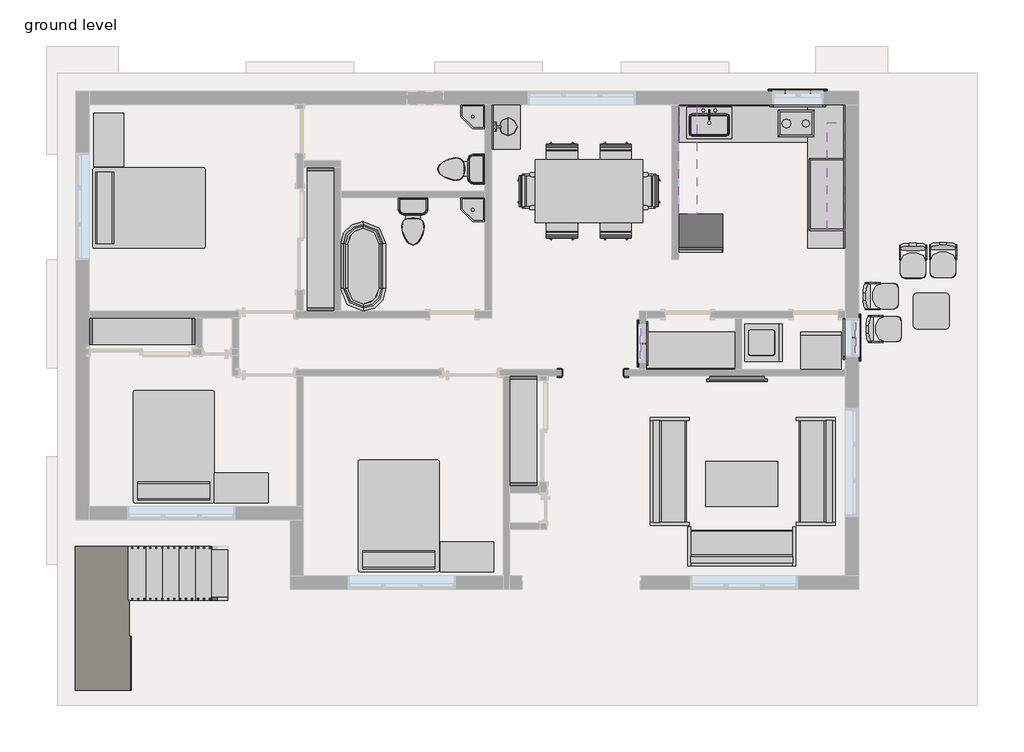
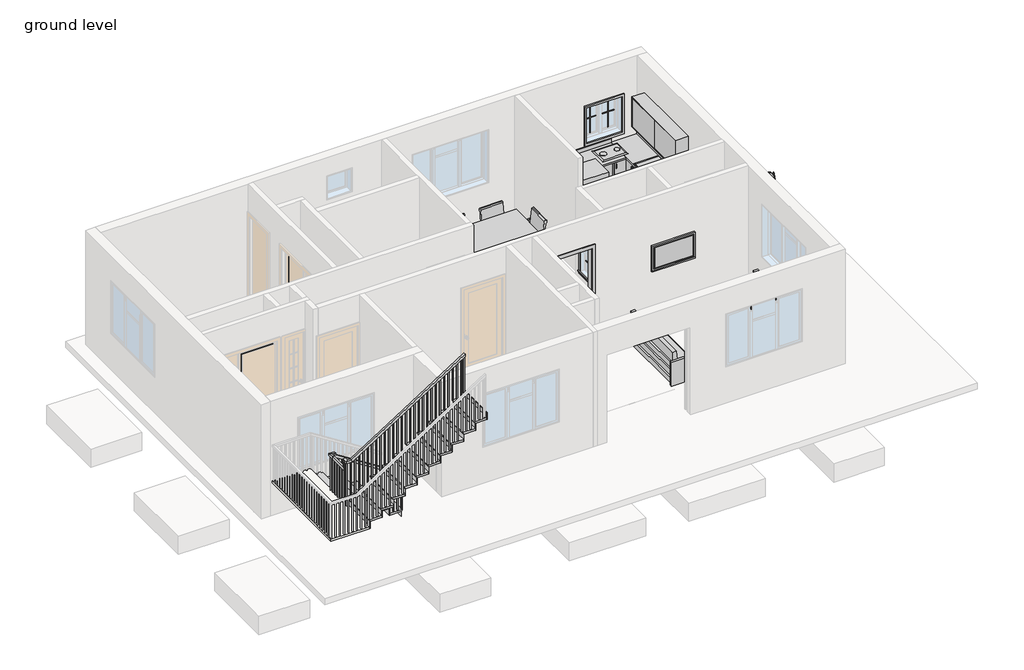
# One storey, part 4 of 4: 34 furniture elements, 17 proxies, 7 flow terminals, 2 stair flights, 1 railing, 1 slab.
# Revit data of these elements (continued)
# Type "Handrail - Rectangular" (continued)
#   built-in parameter 1008604 = 0.166667 (stored number, unit not read)
#   built-in parameter 1008603 = 0.166667 (stored number, unit not read)
#   Railing Height = 3' - 0"
#   built-in parameter 1008630 = 2
#   built-in parameter 1008610 = 2
#   built-in parameter 1008618 = Baluster - Square : 3/4"
# Element 1 (IfcBuildingElementProxy, "Cook Top-2 Unit : 12\" x 18\"")
#   Phase Created = New Construction
#   Materials on its faces: "Metal - Steel, Polished", "Metal - Chrome"
# Element 2 (IfcBuildingElementProxy, "Dryer : 27\" x 25\" x 35\"")
#   Phase Created = New Construction
#   Materials on its faces: "Metal - Paint Finish - Ivory,Glossy"
# Elements 3, 4 (IfcBuildingElementProxy, "Muntin Pattern_2x2 : Muntin Pattern_2x2")
#   Width = 0' - 11 5/8"
#   Height = 2' - 6 1/2"
#   Interior Material = Wood - Stained
#   Exterior Material = Clad - White
#   Phase Created = New Construction
#   Materials on its faces: "Clad - White", "Wood - Stained"
# Elements 5, 6, 7, 8 (IfcBuildingElementProxy, "Muntin Pattern_2x2 : Muntin Pattern_2x2")
#   Width = 1' - 8"
#   Height = 1' - 5 1/8"
#   Interior Material = Wood - Stained
#   Exterior Material = Clad - White
#   Phase Created = New Construction
#   Materials on its faces: "Clad - White", "Wood - Stained"
# Element 9 (IfcBuildingElementProxy, "Passage Opening-Cased : 36\" x 84\"")
#   Phase Created = New Construction
#   Materials on its faces: "Door - Frame"
# Element 10 (IfcBuildingElementProxy, "Refrigerator-Built-in : 30\" x 24\" RH")
#   Phase Created = New Construction
#   Materials on its faces: "Metal - Paint Finish - Ivory,Glossy", "Metal - Chrome"
# Element 11 (IfcBuildingElementProxy, "Trim-Window-Exterior-Flat : with Sill")
#   Opening Width = 2' - 10"
#   Opening Height = 3' - 0"
#   Trim Material = Clad - White
#   Phase Created = New Construction
#   Materials on its faces: "Clad - White"
# Elements 12, 13 (IfcBuildingElementProxy, "Trim-Window-Exterior-Flat : with Sill")
#   Opening Width = 2' - 2"
#   Opening Height = 3' - 6"
#   Trim Material = Clad - White
#   Phase Created = New Construction
#   Materials on its faces: "Clad - White"
# Element 14 (IfcBuildingElementProxy, "Trim-Window-Interior-Flat : Picture Frame")
#   Opening Width = 2' - 10"
#   Opening Height = 3' - 0"
#   Trim Material = Wood - Stained
#   Phase Created = New Construction
#   Materials on its faces: "Wood - Stained"
# Elements 15, 16 (IfcBuildingElementProxy, "Trim-Window-Interior-Flat : Picture Frame")
#   Opening Width = 2' - 2"
#   Opening Height = 3' - 6"
#   Trim Material = Wood - Stained
#   Phase Created = New Construction
#   Materials on its faces: "Wood - Stained"
# Element 17 (IfcBuildingElementProxy, "Washer : 25\" x 25\" x 35\"")
#   Phase Created = New Construction
#   Materials on its faces: "Metal - Paint Finish - Ivory,Matte"
# Element 18 (IfcFlowTerminal, "Lavatory - Vanity : 30\"x18\" - Private")
#   Mark = "6"
#   Flow Pressure = 8.00 psi
#   Phase Created = New Construction
# Element 19 (IfcFlowTerminal, "Sink - Mop : 28\"x28\"")
#   Mark = "4"
#   Phase Created = New Construction
# Element 20 (IfcFlowTerminal, "Sink - Mop : 28\"x28\"")
#   Mark = "5"
#   Phase Created = New Construction
# Element 21 (IfcFlowTerminal, "Sink Kitchen-Single : 30\" x 21\"")
#   Mark = "2"
#   Phase Created = New Construction
#   Materials on its faces: "Steel, Polished"
# Element 22 (IfcFlowTerminal, "Toilet-Domestic-3D : Toilet-Domestic-3D")
#   Mark = "7"
#   Phase Created = New Construction
#   Materials on its faces: "Porcelain, Linen", "Laminate, Linen, Matte"
# Element 23 (IfcFlowTerminal, "Toilet-Domestic-3D : Toilet-Domestic-3D")
#   Mark = "8"
#   Phase Created = New Construction
#   Materials on its faces: "Porcelain, Linen", "Laminate, Linen, Matte"
# Element 24 (IfcFlowTerminal, "Tub-Free Standing-3D : 30\" x 60\"")
#   Mark = "1"
#   Phase Created = New Construction
#   Materials on its faces: "Porcelain, Ivory"
# Element 25 (IfcFurniture, "48\"")
#   Phase Created = New Construction
#   Materials on its faces: "Cabinets", "Cabinets - Handles"
# Element 26 (IfcFurniture, "Base Cabinet-Combo01 : 30\"")
#   Phase Created = New Construction
#   Materials on its faces: "Cabinet"
# Element 27 (IfcFurniture, "Base Cabinet-Corner Unit-Square : 36\"")
#   Phase Created = New Construction
#   Materials on its faces: "Cabinets", "Cabinets - Handles"
# Elements 28, 29, 30 (IfcFurniture, "Bed-Standard : Double 54\" x 75\"")
#   Phase Created = New Construction
#   Materials on its faces: "Linen, White", "Steel, Chrome Plated"
# Elements 31, 32, 33 (IfcFurniture, "Cabinet File-Lateral 2 Drawer : 36\" x 20\" x 24\"")
#   Phase Created = New Construction
#   Materials on its faces: "Metal - Steel"
# Elements 34, 35, 36, 37 (IfcFurniture, "Chair-Task : Chair-Task")
#   Phase Created = New Construction
#   Materials on its faces: "Plastic - Black", "Textile - Slate Blue"
# Elements 38, 39 (IfcFurniture, "Chair-Task Arms : Chair-Task Arms")
#   Phase Created = New Construction
#   Materials on its faces: "Plastic - Black", "Textile - Slate Blue"
# Element 40 (IfcFurniture, "Counter Top : 24\" Depth")
#   Length = 8' - 0"
#   Phase Created = New Construction
#   Materials on its faces: "Counter Top"
# Element 41 (IfcFurniture, "Counter Top : 24\" Depth")
#   Length = 4' - 11 1/2"
#   Phase Created = New Construction
#   Materials on its faces: "Counter Top"
# Element 42 (IfcFurniture, "Counter Top w Sink Hole : 24\" Depth")
#   Sink Opening Width = 2' - 3"
#   Sink Opening Depth = 1' - 3"
#   Sink Location To Wall = 0' - 6"
#   Sink Location = 1' - 8 1/2"
#   Length = 7' - 2 1/4"
#   Phase Created = New Construction
#   Materials on its faces: "Counter Top"
# Elements 43, 44, 45, 46 (IfcFurniture, "Seating-Auditorium : 18\" x 24\" x 30\"")
#   Phase Created = New Construction
#   Materials on its faces: "Steel, Paint Finish, Dark Gray, Matte", "Linen, Beige"
# Element 47 (IfcFurniture, "Shelving : 96\" x 12\" x 84\"")
#   Phase Created = New Construction
#   Materials on its faces: "Laminate, Ivory, Matte"
# Element 48 (IfcFurniture, "Shelving : 96\" x 12\" x 84\" 2")
#   Phase Created = New Construction
#   Materials on its faces: "Laminate, Ivory, Matte"
# Element 49 (IfcFurniture, "Shelving : 96\" x 12\" x 84\" 3")
#   Phase Created = New Construction
#   Materials on its faces: "Laminate, Ivory, Matte"
# Elements 50, 51, 52 (IfcFurniture, "Sofa : 72\"")
#   Phase Created = New Construction
#   Materials on its faces: "Cherry", "Linen, Beige"
# Element 53 (IfcFurniture, "Table-Coffee Rectangular : 48\" x 30\"")
#   Phase Created = New Construction
#   Materials on its faces: "Metal - Chrome", "Glass - Clear, Grey"
# Element 54 (IfcFurniture, "Table-Conference2 w Chairs : 40\" x 90\"")
#   Phase Created = New Construction
#   Materials on its faces: "Wood - Cherry"
# Element 55 (IfcFurniture, "Table-End : 24\" x 24\"")
#   Phase Created = New Construction
#   Materials on its faces: "Laminate, Ivory, Matte", "Birch"
# Element 56 (IfcFurniture, "Television-Plasma : 42\"")
#   Phase Created = New Construction
#   Materials on its faces: "Plastic - Gray", "Glass"
# Elements 57, 58 (IfcFurniture, "Upper Cabinet-Pass-Thru w Glass : 48\" x 30\" x 12\"")
#   Phase Created = New Construction
#   Materials on its faces: "Glass", "Cabinet"
# Element 59 (IfcRailing, "Handrail - Rectangular")
#   Phase Created = New Construction
# Element 60 (IfcSlab, "Non-Monolithic Landing")
#   Phase Created = New Construction
# Elements 61, 62 (IfcStairFlight, "2\" Tread 1\" Nosing 1/4\" Riser")
#   Phase Created = New Construction
# Materials
#   "Metal - Chrome": colour RGB 57 57 57, transparency 0
#   "Metal - Steel, Polished": colour RGB 57 57 57, transparency 0
#   "Metal - Paint Finish - Ivory,Glossy": colour RGB 247 247 239, transparency 0
#   "Door - Frame": colour RGB 118 70 51, transparency 0, Cost = 0
#   "Metal - Paint Finish - Ivory,Matte": colour RGB 247 247 239, transparency 0
#   "Steel, Polished": class "Metal", colour RGB 57 57 57, transparency 0, Description = "Polished steel", Cost = 0
#   "Porcelain, Linen": class "Ceramic", colour RGB 249 239 230, transparency 0, Description = "Porcelain, linen", Cost = 0
#   "Laminate, Linen, Matte": class "Plastic", colour RGB 249 239 230, transparency 0, Description = "Plastic Laminate - Linen, Matte", Cost = 0
#   "Porcelain, Ivory": class "Ceramic", colour RGB 247 247 239, transparency 0, Description = "Porcelain, ivory", Cost = 0
#   "Cabinets - Handles": class "Metal", colour RGB 57 57 57, transparency 0
#   "Cabinets": colour RGB 249 249 249, transparency 0
#   "Steel, Chrome Plated": class "Metal", colour RGB 17 17 17, transparency 0, Description = "Chromiuim plated steel", Cost = 0
#   "Linen, White": class "Textile", colour RGB 247 247 239, transparency 0, Description = "Linen, white", Cost = 0
#   "Metal - Steel": colour RGB 210 210 210, transparency 0
#   "Plastic - Black": colour RGB 0 0 0, transparency 0
#   "Textile - Slate Blue": colour RGB 98 102 118, transparency 0
#   "Linen, Beige": class "Textile", colour RGB 249 239 230, transparency 0, Description = "Linen, beige", Cost = 0
#   "Steel, Paint Finish, Dark Gray, Matte": class "Metal", colour RGB 0 0 0, transparency 0, Description = "Steel, paint finish, dark gray, matte", Cost = 0
#   "Laminate, Ivory, Matte": class "Plastic", colour RGB 247 247 239, transparency 0, Description = "Plastic Laminate - Ivory, Matte", Cost = 0
#   "Cherry": class "Wood", colour RGB 226 177 128, transparency 0, Description = "Prunus Serotina", Cost = 0
#   "Glass - Clear, Grey": colour RGB 252 255 255, transparency 0.64
#   "Wood - Cherry": colour RGB 151 75 0, transparency 0
#   "Birch": class "Wood", colour RGB 224 178 126, transparency 0, Description = "Betula Alleghaniensis", Cost = 0
#   "Plastic - Gray": colour RGB 134 134 134, transparency 0
#   "Clad - White": class "Wood", colour RGB 242 242 238, transparency 0, Cost = 0
#   "Wood - Stained": class "Wood", colour RGB 224 178 126, transparency 0, Cost = 0
#   "Cabinet": colour RGB 204 122 2, transparency 0
#   "Counter Top": class "Wood", colour RGB 226 177 128, transparency 0
#   "Glass": class "Glass", colour RGB 0 128 192, transparency 0.75, Description = "Soda Lime Glass", Cost = 0
